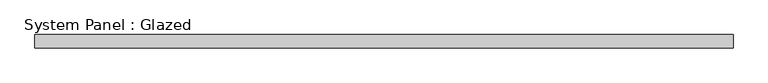
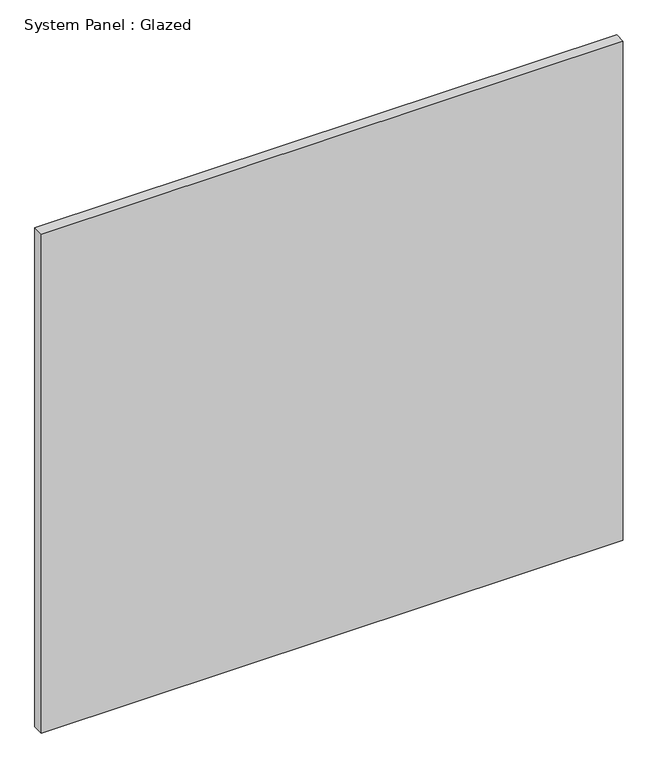
"""IFC4 building model written with IfcOpenShell, lengths in millimetres: plate geometry, System Panel : Glazed."""

from ifc_helpers import new_model, si_unit, origin, origin_with_axes, place, context, project, spatial, polyline, outline, extrude, source, transform, mapped, element, save


def system_panel_glazed_c10ab47a(model_context):
    return source(origin(), model_context, "Body", "SweptSolid", [
        extrude(outline(polyline([(672.6522472, 19.05), (-672.6522472, 19.05), (-672.6522472, 44.45), (672.6522472, 44.45), (672.6522472, 19.05)])), origin_with_axes(), (0.0, 0.0, 1.0), 1219.2),
    ])


if __name__ == "__main__":
    model = new_model("IFC4")
    model_context = context("Model", 3, world=origin())
    ifc_project = project(units=[si_unit("LENGTHUNIT", "METRE", prefix="MILLI")], contexts=[model_context])
    site = spatial("IfcSite", under=ifc_project)
    building = spatial("IfcBuilding", under=site)
    placement = place(None, origin())
    system_panel_glazed_shape = system_panel_glazed_c10ab47a(model_context)
    element("IfcPlate", 1, ObjectType="System Panel : Glazed", at=placement, inside=building, context=model_context, shape_type="MappedRepresentation", body=[
        mapped(system_panel_glazed_shape, transform((0.0, 0.0, 0.0), x_axis=(1.0, 0.0, 0.0), y_axis=(0.0, 1.0, 0.0), z_axis=(0.0, 0.0, 1.0))),
    ])
    save(model, "model.ifc")

# Revit data of these elements
# Type "System Panel : Glazed"
#   Construction Type Id = "GSP4R"
#   Analytic Construction = "1/8 in Pilkington single glazing"
#   Visual Light Transmittance = 0.9
#   Solar Heat Gain Coefficient = 0.86
#   Heat Transfer Coefficient (U) = 1.18115 BTU/(h·ft²·°F)
# Element 1 (IfcPlate, "System Panel : Glazed")
#   Materials on its faces: "Glass"
# Materials
#   "Glass": class "Glass", colour RGB 0 128 192, transparency 0.75, Description = "Soda Lime Glass", Cost = 0
